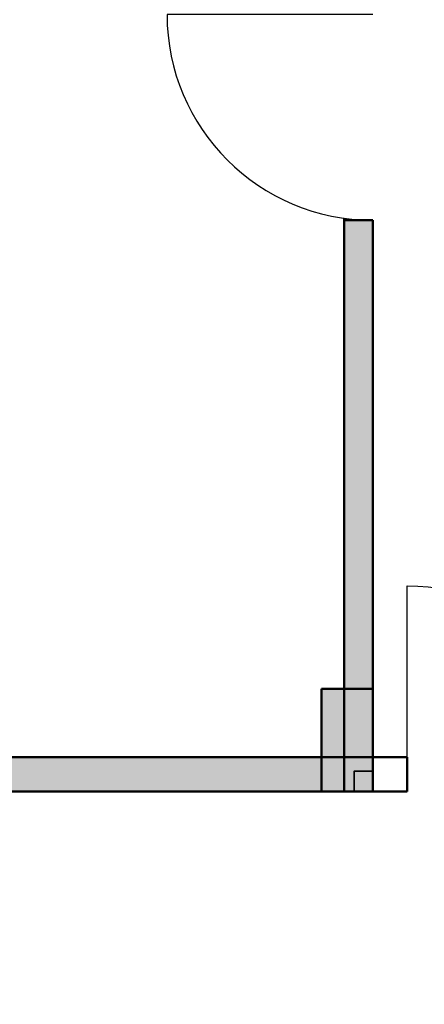
# Model space of a CAD drawing. Units: inches. Extents: x -7 to 1228, y -146 to 1091.
# Tile 69 of 88: x 745 to 816, y 531 to 703. Entities that reach past the tile are written whole.
import ezdxf

# ---------------------------------------------------------------- set-up
doc = ezdxf.new("R2010")
doc.units = ezdxf.units.IN
for name, color, linetype, lineweight in [('A-COLS', 6, 'Continuous', 35), ('A-DOOR', 4, 'Continuous', 25), ('A-WALL', 7, 'Continuous', 50), ('A-WALL-PATT', 251, 'Continuous', 13)]:
    doc.layers.add(name, color=color, linetype=linetype, lineweight=lineweight)

# ---------------------------------------------------------------- blocks, each defined once
blk = doc.blocks.new('DOOR-900')
blk.add_line((36, 0), (36, 36))
blk.add_arc((36, 0), 36, 90, 180)

msp = doc.modelspace()

# ---------------------------------------------------------------- hatches: boundary and pattern name
at = {"layer": 'A-COLS'}
h = msp.add_hatch(color=256, dxfattribs=at)
h.dxf.hatch_style = 1
h.paths.add_polyline_path([(807, 586), (798, 586), (798, 568), (803.71, 568), (803.71, 571.55), (807, 571.55)])
h = msp.add_hatch(color=256, dxfattribs=at)
h.dxf.hatch_style = 1
h.paths.add_polyline_path([(803.71, 571.55), (803.71, 568), (807, 568), (807, 571.55)])
at = {"layer": 'A-WALL-PATT'}
h = msp.add_hatch(color=256, dxfattribs=at)
h.dxf.hatch_style = 1
h.paths.add_polyline_path([(69, 568), (60, 568), (60, 493), (63.29, 493), (69, 493)])
h.paths.add_polyline_path([(69, 662.41), (60, 662.41), (60, 586), (69, 586)], flags=17)
h.paths.add_polyline_path([(69, 723), (184, 723), (184, 734), (179, 734), (179, 728), (69, 728), (69, 741.62), (60, 741.62), (60, 698.41), (69, 698.41)], flags=17)
h.paths.add_polyline_path([(69, 782), (231, 782), (231, 728), (231, 723), (231, 586), (236, 586), (236, 787), (69, 787), (69, 800.13), (60, 800.13), (60, 765.62), (69, 765.62)])
h.paths.add_polyline_path([(184, 842), (189, 842), (189, 848), (173, 848), (173, 842), (179, 842), (179, 787), (184, 787)])
h.paths.add_polyline_path([(118.22, 69), (69, 69), (69, 60), (118.22, 60)])
h.paths.add_polyline_path([(227, 69), (154.22, 69), (154.22, 60), (227, 60)])
h.paths.add_polyline_path([(236, 60), (232.71, 60), (227, 60), (227, 36), (236, 36)])
h.paths.add_polyline_path([(389, 60), (380, 60), (380, 36), (389, 36)])
h.paths.add_polyline_path([(384, 181), (380, 181), (380, 115), (380, 78), (384, 78)])
h.paths.add_polyline_path([(380, 115), (334.55, 115), (334.55, 109), (380, 109)])
h.paths.add_polyline_path([(274.55, 115), (236, 115), (236, 201), (232.71, 201), (231, 201), (231, 78), (236, 78), (236, 109), (274.55, 109)])
h.paths.add_polyline_path([(69, 123), (60, 123), (60, 78), (69, 78)])
h.paths.add_polyline_path([(69, 201), (60, 201), (60, 159), (69, 159)])
h.paths.add_polyline_path([(143, 219), (69, 219), (69, 213), (143, 213)], flags=17)
h.paths.add_polyline_path([(189, 219), (184, 219), (184, 274), (231, 274), (231, 219), (236, 219), (236, 279), (184, 279), (184, 297), (179, 297), (179, 279), (69, 279), (69, 290.91), (60, 290.91), (60, 262.18), (69, 262.18), (69, 274), (179, 274), (179, 219), (173, 219), (173, 213), (189, 213)])
h.paths.add_polyline_path([(69, 238.18), (60, 238.18), (60, 219), (69, 219)], flags=17)
h.paths.add_polyline_path([(69, 333), (60, 333), (60, 314.91), (69, 314.91), (69, 316.96)])
h.paths.add_polyline_path([(190, 338), (184, 338), (69, 338), (69, 333), (179, 333), (179, 327), (184, 327), (184, 333.02), (190, 333.05)])
h.paths.add_polyline_path([(69, 386.81), (60, 386.81), (60, 351), (69, 351)])
h.paths.add_polyline_path([(69, 475), (60, 475), (60, 422.81), (69, 422.81)])
h.paths.add_polyline_path([(236, 475), (231, 475), (231, 351.24), (236, 351.24)])
h.paths.add_polyline_path([(384, 475), (380, 475), (380, 362), (384, 362)])
h.paths.add_polyline_path([(547, 307), (439, 307), (439, 356), (445, 356), (445, 362), (433, 362), (433, 307), (380, 307), (380, 244), (380, 241), (384, 241), (384, 301), (433, 301), (433, 277), (439, 277), (439, 301), (547, 301)])
h.paths.add_polyline_path([(547, 241), (439, 241), (439, 247), (433, 247), (433, 235), (547, 235)])
h.paths.add_polyline_path([(450, 69), (440.29, 69), (424.89, 69), (389, 69), (389, 60), (450, 60)])
h.paths.add_polyline_path([(547, 69), (486, 69), (486, 60), (547, 60)])
h.paths.add_polyline_path([(556, 148.27), (547, 148.27), (547, 78), (556, 78)])
h.paths.add_polyline_path([(556, 223), (547, 223), (547, 195), (547, 184.27), (556, 184.27)])
h.paths.add_polyline_path([(556, 311.19), (547, 311.19), (547, 273.08), (556, 273.08)])
h.paths.add_polyline_path([(556, 344), (552.71, 344), (547, 344), (547, 335.19), (556, 335.19)])
h.paths.add_polyline_path([(556, 249.08), (547, 249.08), (547, 241), (556, 241)])
h.paths.add_polyline_path([(547, 362), (475, 362), (475, 356), (547, 356)], flags=0)
h.paths.add_polyline_path([(556, 399.62), (547, 399.62), (547, 362), (556, 362)])
h.paths.add_polyline_path([(556, 475), (547, 475), (547, 435.62), (556, 435.62)])
h.paths.add_polyline_path([(547, 493), (389, 493), (389, 487), (547, 487)])
h.paths.add_polyline_path([(380, 493), (278, 493), (278, 487), (380, 487)])
h.paths.add_polyline_path([(227, 493), (69, 493), (69, 487), (227, 487)])
h.paths.add_polyline_path([(643, 122.44), (634, 122.44), (634, 78), (643, 78)])
h.paths.add_polyline_path([(702.5, 69), (692.79, 69), (677.39, 69), (643, 69), (643, 60), (702.5, 60)])
h.paths.add_polyline_path([(798, 69), (738.5, 69), (738.5, 60), (798, 60)])
h.paths.add_polyline_path([(807, 60), (803.71, 60), (798, 60), (798, 36), (807, 36)])
h.paths.add_polyline_path([(807, 109), (846.75, 109), (846.75, 115), (807, 115), (807, 159), (802, 159), (802, 78), (807, 78)])
h.paths.add_polyline_path([(807, 201), (802, 201), (802, 195), (807, 195)])
h.paths.add_polyline_path([(643, 201), (634, 201), (634, 158.44), (643, 158.44)])
h.paths.add_polyline_path([(756, 225), (751, 225), (751, 219), (643, 219), (643, 213), (756, 213)])
h.paths.add_polyline_path([(643, 240.85), (634, 240.85), (634, 219), (643, 219)])
h.paths.add_polyline_path([(643, 274), (643, 288.63), (634, 288.63), (634, 264.85), (643, 264.85)])
h.paths.add_polyline_path([(802, 279), (756, 279), (756, 297), (751, 297), (751, 279), (643, 279), (643, 274), (751, 274), (751, 255), (756, 255), (756, 274), (802, 274)])
h.paths.add_polyline_path([(807, 333), (803.71, 333), (802, 333), (802, 279), (802, 274), (802, 219), (807, 219)])
h.paths.add_polyline_path([(956, 182), (951, 182), (951, 115), (906.75, 115), (906.75, 109), (951, 109), (951, 78), (956, 78)])
h.paths.add_polyline_path([(960, 60), (951, 60), (951, 36), (960, 36)])
h.paths.add_polyline_path([(1021, 69), (1005.78, 69), (960, 69), (960, 60), (1021, 60)])
h.paths.add_polyline_path([(956, 224), (951, 224), (951, 218), (956, 218)])
h.paths.add_polyline_path([(956, 302), (1004, 302), (1004, 278), (1010, 278), (1010, 302), (1118, 302), (1118, 290.81), (1127, 290.81), (1127, 326.97), (1118, 326.97), (1118, 320.97), (1118, 307), (1010, 307), (1010, 356), (1016, 356), (1016, 362), (1004, 362), (1004, 307), (951, 307), (951, 244), (951, 242), (954.29, 242), (956, 242)])
h.paths.add_polyline_path([(643, 333), (634, 333), (634, 312.63), (643, 312.63), (643, 316.96)])
h.paths.add_polyline_path([(756, 338), (643, 338), (643, 333), (751, 333), (751, 327), (756, 327)])
h.paths.add_polyline_path([(643, 388), (634, 388), (634, 351), (643, 351)])
h.paths.add_polyline_path([(807, 357), (802, 357), (802, 351), (807, 351)])
h.paths.add_polyline_path([(807, 475), (802, 475), (802, 393), (807, 393)])
h.paths.add_polyline_path([(643, 475), (634, 475), (634, 424), (643, 424)])
h.paths.add_polyline_path([(798, 493), (643, 493), (643, 487), (798, 487)])
h.paths.add_polyline_path([(634, 493), (556, 493), (556, 487), (634, 487)])
h.paths.add_polyline_path([(813, 493), (807, 493), (807, 487), (813, 487)])
h.paths.add_polyline_path([(951, 493), (849, 493), (849, 487), (951, 487)])
h.paths.add_polyline_path([(956, 484), (951, 484), (951, 374), (956, 374)])
h.paths.add_polyline_path([(1109, 493), (969, 493), (969, 487), (1109, 487)])
h.paths.add_polyline_path([(1127, 484), (1118, 484), (1118, 450.64), (1127, 450.64)])
h.paths.add_polyline_path([(1127, 414.64), (1118, 414.64), (1118, 365), (1127, 365)])
h.paths.add_polyline_path([(1109, 362), (1046, 362), (1046, 356), (1109, 356)], flags=17)
h.paths.add_polyline_path([(1127, 356), (1123.45, 356), (1118, 356), (1118, 350.97), (1127, 350.97)], flags=0)
h.paths.add_polyline_path([(1127, 266.81), (1118, 266.81), (1118, 262.36), (1118, 242), (1127, 242)], flags=17)
h.paths.add_polyline_path([(1118, 242), (1010, 242), (1010, 248), (1004, 248), (1004, 237), (1118, 237)])
h.paths.add_polyline_path([(1127, 224), (1118, 224), (1118, 170), (1127, 170)])
h.paths.add_polyline_path([(1127, 134), (1118, 134), (1118, 78), (1127, 78)])
h.paths.add_polyline_path([(1118, 69), (1057, 69), (1057, 60), (1118, 60)])
h.paths.add_polyline_path([(227, 571.55), (227, 574), (69, 574), (69, 568), (227, 568)])
h.paths.add_polyline_path([(380, 571.55), (380, 574), (278, 574), (278, 568), (380, 568)])
h.paths.add_polyline_path([(242, 574), (236, 574), (236, 568), (242, 568)])
h.paths.add_polyline_path([(547, 571.55), (547, 574), (389, 574), (389, 568), (547, 568)])
h.paths.add_polyline_path([(384, 733), (380, 733), (380, 586), (384, 586)])
h.paths.add_polyline_path([(556, 646), (634, 646), (634, 655), (547, 655), (547, 586), (556, 586)])
h.paths.add_polyline_path([(634, 574), (556, 574), (556, 568), (634, 568)])
h.paths.add_polyline_path([(643, 655), (634, 655), (634, 586), (643, 586)])
h.paths.add_polyline_path([(798, 574), (643, 574), (643, 568), (798, 568)])
h.paths.add_polyline_path([(643, 663.85), (634, 663.85), (634, 655), (643, 655)])
h.paths.add_polyline_path([(556, 676.97), (547, 676.97), (547, 655), (556, 655)])
h.paths.add_polyline_path([(556, 733), (547, 733), (547, 712.97), (556, 712.97)])
h.paths.add_polyline_path([(643, 710), (634, 710), (634, 699.85), (643, 699.85)])
h.paths.add_polyline_path([(807, 668), (802, 668), (802, 586), (807, 586)])
h.paths.add_polyline_path([(951, 574), (849, 574), (849, 568), (951, 568)])
h.paths.add_polyline_path([(956, 691), (951, 691), (951, 577), (956, 577)])
h.paths.add_polyline_path([(1109, 574), (969, 574), (969, 568), (1109, 568)])
h.paths.add_polyline_path([(1127, 643.4), (1118, 643.4), (1118, 577), (1127, 577)])
h.paths.add_polyline_path([(1127, 568), (1123.45, 568), (1118, 568), (1118, 493), (1127, 493)])
h.paths.add_polyline_path([(1127, 733), (1118, 733), (1118, 679.4), (1127, 679.4)])
h.paths.add_polyline_path([(1127, 777.35), (1118, 777.35), (1118, 770.04), (1118, 751), (1127, 751)], flags=17)
h.paths.add_polyline_path([(1118, 751), (1010, 751), (1010, 757), (1004, 757), (1004, 745), (1118, 745)])
h.paths.add_polyline_path([(956, 811), (1004, 811), (1004, 787), (1010, 787), (1010, 811), (1017.87, 811), (1017.87, 811.63, -0.414214), (1018.25, 812), (1031.98, 812, -0.414214), (1032.35, 811.63), (1032.35, 811), (1118, 811), (1118, 801.35), (1127, 801.35), (1127, 834.69), (1118, 834.69), (1118, 830.24), (1118, 817), (1010, 817), (1010, 866), (1016, 866), (1016, 872), (1004, 872), (1004, 817), (956, 817), (956, 866), (951, 866), (951, 751), (954.29, 751), (956, 751)])
h.paths.add_polyline_path([(1118, 872), (1046, 872), (1046, 866), (1118, 866)], flags=17)
h.paths.add_polyline_path([(1127, 924.71), (1118, 924.71), (1118, 884), (1127, 884)])
h.paths.add_polyline_path([(1127, 866), (1123.71, 866), (1118, 866), (1118, 858.69), (1127, 858.69)], flags=17)
h.paths.add_polyline_path([(956, 983), (951, 983), (951, 952), (807, 952), (807, 983), (802, 983), (802, 902), (807, 902), (807, 946), (951, 946), (951, 884), (956, 884)])
h.paths.add_polyline_path([(807, 842), (802, 842), (802, 787), (756, 787), (756, 806), (751, 806), (751, 787), (643, 787), (643, 782), (751, 782), (751, 764), (756, 764), (756, 782), (802, 782), (802, 728), (807, 728)])
h.paths.add_polyline_path([(756, 848), (643, 848), (643, 842), (751, 842), (751, 836), (756, 836)])
h.paths.add_polyline_path([(756, 734), (751, 734), (751, 728), (643, 728), (643, 723), (756, 723)])
h.paths.add_polyline_path([(643, 749.79), (634, 749.79), (634, 728), (637.29, 728), (643, 728)])
h.paths.add_polyline_path([(643, 805.41), (634, 805.41), (634, 773.79), (643, 773.79)])
h.paths.add_polyline_path([(643, 896.66), (634, 896.66), (634, 860), (637.29, 860), (643, 860)])
h.paths.add_polyline_path([(643, 842), (634, 842), (634, 829.41), (643, 829.41)])
h.paths.add_polyline_path([(643, 983), (634, 983), (634, 932.66), (643, 932.66)])
h.paths.add_polyline_path([(1127, 983), (1118, 983), (1118, 960.71), (1127, 960.71)])
h.paths.add_polyline_path([(1118, 1001), (1077.53, 1001), (1077.53, 992), (1118, 992)])
h.paths.add_polyline_path([(1041.53, 1001), (960, 1001), (960, 992), (1041.53, 992)])
h.paths.add_polyline_path([(960, 1025), (951, 1025), (951, 1001), (954.29, 1001), (960, 1001)])
h.paths.add_polyline_path([(807, 1025), (798, 1025), (798, 1001), (807, 1001)])
h.paths.add_polyline_path([(798, 1001), (738.5, 1001), (738.5, 992), (798, 992)])
h.paths.add_polyline_path([(702.5, 1001), (643, 1001), (643, 992), (702.5, 992)])
h.paths.add_polyline_path([(547, 1001), (499.11, 1001), (499.11, 992), (547, 992)])
h.paths.add_polyline_path([(463.11, 1001), (389, 1001), (389, 992), (463.11, 992)])
h.paths.add_polyline_path([(389, 1025), (380, 1025), (380, 1022), (380, 1001), (383.29, 1001), (389, 1001)])
h.paths.add_polyline_path([(236, 1025), (227, 1025), (227, 1001), (236, 1001)])
h.paths.add_polyline_path([(236, 983), (231, 983), (231, 860), (236, 860)])
h.paths.add_polyline_path([(274.55, 952), (236, 952), (236, 946), (274.55, 946)])
h.paths.add_polyline_path([(380, 952), (334.55, 952), (334.55, 946), (380, 946)])
h.paths.add_polyline_path([(384, 983), (380, 983), (380, 884), (383.29, 884), (384, 884)])
h.paths.add_polyline_path([(227, 1001), (155.01, 1001), (155.01, 992), (162.87, 992), (227, 992)])
h.paths.add_polyline_path([(119.01, 1001), (69, 1001), (69, 992), (119.01, 992)])
h.paths.add_polyline_path([(69, 983), (60, 983), (60, 922.99), (69, 922.99)])
h.paths.add_polyline_path([(69, 886.99), (60, 886.99), (60, 860), (63.29, 860), (69, 860)])
h.paths.add_polyline_path([(143, 848), (69, 848), (69, 842), (143, 842)])

# ---------------------------------------------------------------- linework, layer by layer
at = {"layer": 'A-COLS'}
msp.add_lwpolyline([(807, 568), (803.71, 568), (803.71, 571.55), (807, 571.55)], close=True, dxfattribs=at)
at = {"layer": 'A-WALL'}
for p, q in [((802, 568), (802, 668.35)), ((807, 668), (802, 668)), ((802, 668), (802, 568)), ((807, 668), (807, 568)), ((807, 568), (807, 668)), ((798, 568), (798, 586)), ((798, 586), (807, 586)), ((807, 586), (807, 568)), ((813, 574), (556, 574)), ((807, 568), (807, 574)), ((813, 568), (813, 574)), ((813, 568), (556, 568)), ((807, 568), (798, 568))]:
    msp.add_line(p, q, dxfattribs=at)

# ---------------------------------------------------------------- block references
at = {"layer": 'A-DOOR', "rotation": 89.99999999999964}
msp.add_blockref('DOOR-900', (807, 668), dxfattribs=at)
at = {"layer": 'A-DOOR', "extrusion": (0, 0, -1), "zscale": -1}
msp.add_blockref('DOOR-900', (-849, 568), dxfattribs=at)

doc.saveas('drawing.dxf')
